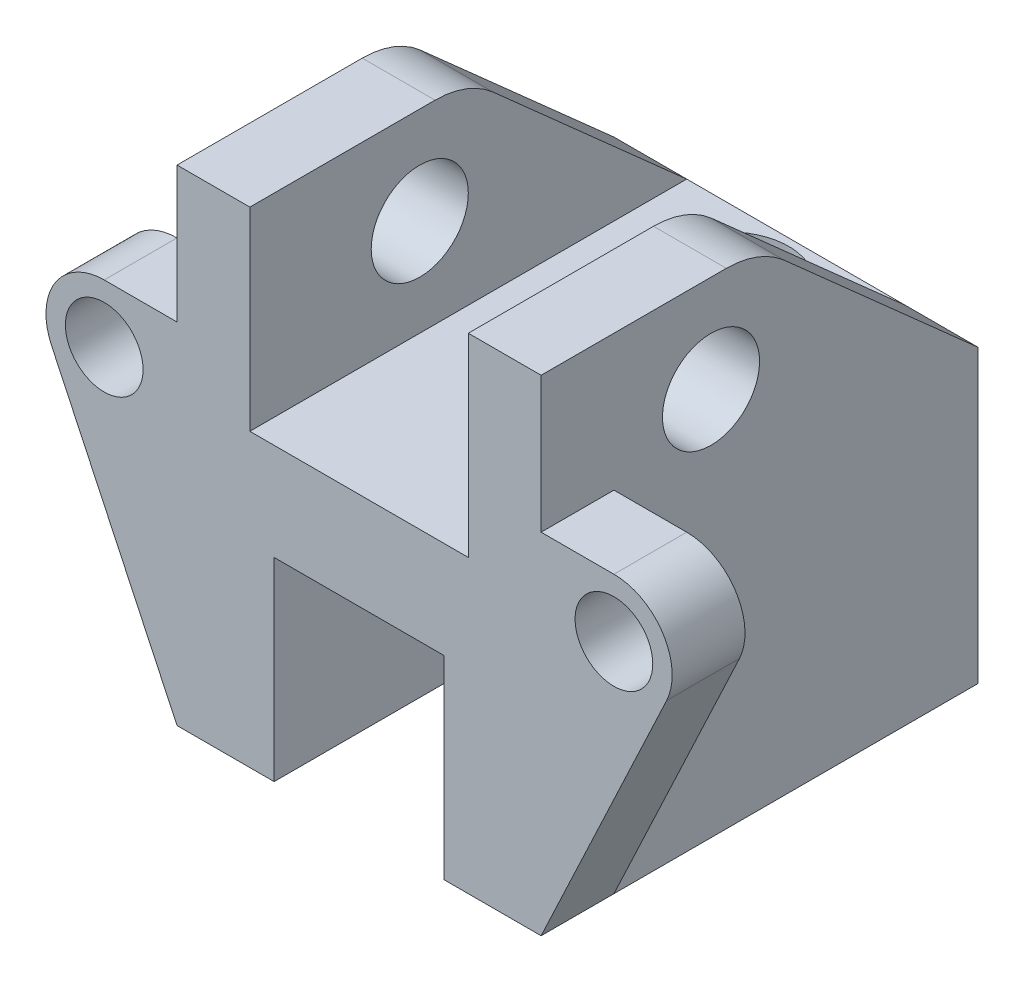
ISO-10303-21;
HEADER;
FILE_DESCRIPTION(('STEP AP214'),'2;1');
FILE_NAME('part.step','',(''),(''),'','','');
FILE_SCHEMA(('AUTOMOTIVE_DESIGN { 1 0 10303 214 1 1 1 1 }'));
ENDSEC;
DATA;
#1=APPLICATION_CONTEXT('core data for automotive mechanical design processes');
#2=APPLICATION_PROTOCOL_DEFINITION('international standard','automotive_design',2000,#1);
#3=PRODUCT_CONTEXT('',#1,'mechanical');
#4=PRODUCT('Part','Part','',(#3));
#5=PRODUCT_RELATED_PRODUCT_CATEGORY('part','',(#4));
#6=PRODUCT_DEFINITION_FORMATION('','',#4);
#7=PRODUCT_DEFINITION_CONTEXT('part definition',#1,'design');
#8=PRODUCT_DEFINITION('design','',#6,#7);
#9=PRODUCT_DEFINITION_SHAPE('','',#8);
#10=(LENGTH_UNIT() NAMED_UNIT(*) SI_UNIT(.MILLI.,.METRE.));
#11=(NAMED_UNIT(*) PLANE_ANGLE_UNIT() SI_UNIT($,.RADIAN.));
#12=(NAMED_UNIT(*) SI_UNIT($,.STERADIAN.) SOLID_ANGLE_UNIT());
#13=UNCERTAINTY_MEASURE_WITH_UNIT(LENGTH_MEASURE(1.E-05),#10,'distance_accuracy_value','');
#14=(GEOMETRIC_REPRESENTATION_CONTEXT(3) GLOBAL_UNCERTAINTY_ASSIGNED_CONTEXT((#13)) GLOBAL_UNIT_ASSIGNED_CONTEXT((#10,
#11,#12)) REPRESENTATION_CONTEXT('',''));
#15=CARTESIAN_POINT('',(0.,0.,0.));
#16=DIRECTION('',(0.,0.,1.));
#17=DIRECTION('',(1.,0.,0.));
#18=AXIS2_PLACEMENT_3D('',#15,#16,#17);
#19=CARTESIAN_POINT('',(-75.,0.,0.));
#20=DIRECTION('',(-1.,0.,0.));
#21=DIRECTION('',(0.,0.,1.));
#22=AXIS2_PLACEMENT_3D('',#19,#20,#21);
#23=PLANE('',#22);
#24=CARTESIAN_POINT('',(-75.,80.,-35.));
#25=DIRECTION('',(1.,0.,0.));
#26=DIRECTION('',(0.,0.,-1.));
#27=AXIS2_PLACEMENT_3D('',#24,#25,#26);
#28=CIRCLE('',#27,10.);
#29=CARTESIAN_POINT('',(-75.,80.,-45.));
#30=VERTEX_POINT('',#29);
#31=EDGE_CURVE('E275',#30,#30,#28,.T.);
#32=ORIENTED_EDGE('',*,*,#31,.T.);
#33=EDGE_LOOP('',(#32));
#34=FACE_BOUND('',#33,.T.);
#35=DIRECTION('',(0.,0.,-1.));
#36=VECTOR('',#35,1.);
#37=CARTESIAN_POINT('',(-75.,0.,0.));
#38=LINE('',#37,#36);
#39=CARTESIAN_POINT('',(-75.,0.,-15.));
#40=VERTEX_POINT('',#39);
#41=CARTESIAN_POINT('',(-75.,0.,-90.));
#42=VERTEX_POINT('',#41);
#43=EDGE_CURVE('E335',#40,#42,#38,.T.);
#44=ORIENTED_EDGE('',*,*,#43,.F.);
#45=DIRECTION('',(0.,1.,0.));
#46=VECTOR('',#45,1.);
#47=CARTESIAN_POINT('',(-75.,72.,-15.));
#48=LINE('',#47,#46);
#49=CARTESIAN_POINT('',(-75.,72.,-15.));
#50=VERTEX_POINT('',#49);
#51=EDGE_CURVE('E216',#40,#50,#48,.T.);
#52=ORIENTED_EDGE('',*,*,#51,.T.);
#53=DIRECTION('',(0.,0.,1.));
#54=VECTOR('',#53,1.);
#55=CARTESIAN_POINT('',(-75.,72.,-15.));
#56=LINE('',#55,#54);
#57=CARTESIAN_POINT('',(-75.,72.,0.));
#58=VERTEX_POINT('',#57);
#59=EDGE_CURVE('E206',#50,#58,#56,.T.);
#60=ORIENTED_EDGE('',*,*,#59,.T.);
#61=DIRECTION('',(0.,-1.,0.));
#62=VECTOR('',#61,1.);
#63=CARTESIAN_POINT('',(-75.,0.,0.));
#64=LINE('',#63,#62);
#65=CARTESIAN_POINT('',(-75.,100.,0.));
#66=VERTEX_POINT('',#65);
#67=EDGE_CURVE('E328',#66,#58,#64,.T.);
#68=ORIENTED_EDGE('',*,*,#67,.F.);
#69=DIRECTION('',(0.,0.,1.));
#70=VECTOR('',#69,1.);
#71=CARTESIAN_POINT('',(-75.,100.,0.));
#72=LINE('',#71,#70);
#73=CARTESIAN_POINT('',(-75.,100.,-38.1564121977173));
#74=VERTEX_POINT('',#73);
#75=EDGE_CURVE('E343',#74,#66,#72,.T.);
#76=ORIENTED_EDGE('',*,*,#75,.F.);
#77=CARTESIAN_POINT('',(-75.,82.,-38.1564121977173));
#78=DIRECTION('',(-1.,0.,0.));
#79=DIRECTION('',(0.,0.,1.));
#80=AXIS2_PLACEMENT_3D('',#77,#78,#79);
#81=CIRCLE('',#80,18.);
#82=CARTESIAN_POINT('',(-75.,95.4533677363059,-50.1149612966559));
#83=VERTEX_POINT('',#82);
#84=EDGE_CURVE('E11',#74,#83,#81,.T.);
#85=ORIENTED_EDGE('',*,*,#84,.T.);
#86=DIRECTION('',(0.,0.66436383882992,0.74740931868366));
#87=VECTOR('',#86,1.);
#88=CARTESIAN_POINT('',(-75.,100.,-45.));
#89=LINE('',#88,#87);
#90=CARTESIAN_POINT('',(-75.,60.,-90.));
#91=VERTEX_POINT('',#90);
#92=EDGE_CURVE('E338',#91,#83,#89,.T.);
#93=ORIENTED_EDGE('',*,*,#92,.F.);
#94=DIRECTION('',(0.,1.,0.));
#95=VECTOR('',#94,1.);
#96=CARTESIAN_POINT('',(-75.,0.,-90.));
#97=LINE('',#96,#95);
#98=EDGE_CURVE('E339',#42,#91,#97,.T.);
#99=ORIENTED_EDGE('',*,*,#98,.F.);
#100=EDGE_LOOP('',(#44,#52,#60,#68,#76,#85,#93,#99));
#101=FACE_BOUND('',#100,.T.);
#102=ADVANCED_FACE('F44',(#34,#101),#23,.T.);
#103=CARTESIAN_POINT('',(0.,0.,0.));
#104=DIRECTION('',(-1.,0.,0.));
#105=DIRECTION('',(0.,0.,1.));
#106=AXIS2_PLACEMENT_3D('',#103,#104,#105);
#107=PLANE('',#106);
#108=CARTESIAN_POINT('',(0.,80.,-35.));
#109=DIRECTION('',(1.,0.,0.));
#110=DIRECTION('',(0.,0.,-1.));
#111=AXIS2_PLACEMENT_3D('',#108,#109,#110);
#112=CIRCLE('',#111,10.);
#113=CARTESIAN_POINT('',(0.,80.,-45.));
#114=VERTEX_POINT('',#113);
#115=EDGE_CURVE('E271',#114,#114,#112,.T.);
#116=ORIENTED_EDGE('',*,*,#115,.F.);
#117=EDGE_LOOP('',(#116));
#118=FACE_BOUND('',#117,.T.);
#119=DIRECTION('',(0.,0.,1.));
#120=VECTOR('',#119,1.);
#121=CARTESIAN_POINT('',(0.,72.,-15.));
#122=LINE('',#121,#120);
#123=CARTESIAN_POINT('',(0.,72.,-15.));
#124=VERTEX_POINT('',#123);
#125=CARTESIAN_POINT('',(0.,72.,0.));
#126=VERTEX_POINT('',#125);
#127=EDGE_CURVE('E263',#124,#126,#122,.T.);
#128=ORIENTED_EDGE('',*,*,#127,.F.);
#129=DIRECTION('',(0.,-1.,0.));
#130=VECTOR('',#129,1.);
#131=CARTESIAN_POINT('',(0.,72.,-15.));
#132=LINE('',#131,#130);
#133=CARTESIAN_POINT('',(0.,0.,-15.));
#134=VERTEX_POINT('',#133);
#135=EDGE_CURVE('E248',#124,#134,#132,.T.);
#136=ORIENTED_EDGE('',*,*,#135,.T.);
#137=DIRECTION('',(0.,0.,-1.));
#138=VECTOR('',#137,1.);
#139=CARTESIAN_POINT('',(0.,0.,0.));
#140=LINE('',#139,#138);
#141=CARTESIAN_POINT('',(0.,0.,-90.));
#142=VERTEX_POINT('',#141);
#143=EDGE_CURVE('E346',#134,#142,#140,.T.);
#144=ORIENTED_EDGE('',*,*,#143,.T.);
#145=DIRECTION('',(0.,1.,0.));
#146=VECTOR('',#145,1.);
#147=CARTESIAN_POINT('',(0.,0.,-90.));
#148=LINE('',#147,#146);
#149=CARTESIAN_POINT('',(0.,60.,-90.));
#150=VERTEX_POINT('',#149);
#151=EDGE_CURVE('E352',#142,#150,#148,.T.);
#152=ORIENTED_EDGE('',*,*,#151,.T.);
#153=DIRECTION('',(0.,0.66436383882992,0.74740931868366));
#154=VECTOR('',#153,1.);
#155=CARTESIAN_POINT('',(0.,100.,-45.));
#156=LINE('',#155,#154);
#157=CARTESIAN_POINT('',(0.,95.4533677363059,-50.1149612966559));
#158=VERTEX_POINT('',#157);
#159=EDGE_CURVE('E351',#150,#158,#156,.T.);
#160=ORIENTED_EDGE('',*,*,#159,.T.);
#161=CARTESIAN_POINT('',(0.,82.,-38.1564121977173));
#162=DIRECTION('',(-1.,0.,0.));
#163=DIRECTION('',(0.,0.,1.));
#164=AXIS2_PLACEMENT_3D('',#161,#162,#163);
#165=CIRCLE('',#164,18.);
#166=CARTESIAN_POINT('',(0.,100.,-38.1564121977173));
#167=VERTEX_POINT('',#166);
#168=EDGE_CURVE('E381',#158,#167,#165,.F.);
#169=ORIENTED_EDGE('',*,*,#168,.T.);
#170=DIRECTION('',(0.,0.,1.));
#171=VECTOR('',#170,1.);
#172=CARTESIAN_POINT('',(0.,100.,0.));
#173=LINE('',#172,#171);
#174=CARTESIAN_POINT('',(0.,100.,0.));
#175=VERTEX_POINT('',#174);
#176=EDGE_CURVE('E334',#167,#175,#173,.T.);
#177=ORIENTED_EDGE('',*,*,#176,.T.);
#178=DIRECTION('',(0.,-1.,0.));
#179=VECTOR('',#178,1.);
#180=CARTESIAN_POINT('',(0.,0.,0.));
#181=LINE('',#180,#179);
#182=EDGE_CURVE('E325',#175,#126,#181,.T.);
#183=ORIENTED_EDGE('',*,*,#182,.T.);
#184=EDGE_LOOP('',(#128,#136,#144,#152,#160,#169,#177,#183));
#185=FACE_BOUND('',#184,.T.);
#186=ADVANCED_FACE('F450',(#118,#185),#107,.F.);
#187=CARTESIAN_POINT('',(-75.,100.,0.));
#188=DIRECTION('',(0.,1.,0.));
#189=DIRECTION('',(0.,0.,1.));
#190=AXIS2_PLACEMENT_3D('',#187,#188,#189);
#191=PLANE('',#190);
#192=DIRECTION('',(0.,0.,1.));
#193=VECTOR('',#192,1.);
#194=CARTESIAN_POINT('',(-60.,100.,0.));
#195=LINE('',#194,#193);
#196=CARTESIAN_POINT('',(-60.,100.,-38.1564121977173));
#197=VERTEX_POINT('',#196);
#198=CARTESIAN_POINT('',(-60.,100.,0.));
#199=VERTEX_POINT('',#198);
#200=EDGE_CURVE('E278',#197,#199,#195,.T.);
#201=ORIENTED_EDGE('',*,*,#200,.F.);
#202=DIRECTION('',(1.,0.,0.));
#203=VECTOR('',#202,1.);
#204=CARTESIAN_POINT('',(-75.,100.,-38.1564121977173));
#205=LINE('',#204,#203);
#206=EDGE_CURVE('E53',#197,#74,#205,.F.);
#207=ORIENTED_EDGE('',*,*,#206,.T.);
#208=ORIENTED_EDGE('',*,*,#75,.T.);
#209=DIRECTION('',(1.,0.,0.));
#210=VECTOR('',#209,1.);
#211=CARTESIAN_POINT('',(-75.,100.,0.));
#212=LINE('',#211,#210);
#213=EDGE_CURVE('E358',#66,#199,#212,.T.);
#214=ORIENTED_EDGE('',*,*,#213,.T.);
#215=EDGE_LOOP('',(#201,#207,#208,#214));
#216=FACE_BOUND('',#215,.T.);
#217=ADVANCED_FACE('F396',(#216),#191,.T.);
#218=CARTESIAN_POINT('',(-75.,100.,-45.));
#219=DIRECTION('',(0.,0.74740931868366,-0.66436383882992));
#220=DIRECTION('',(0.,0.66436383882992,0.74740931868366));
#221=AXIS2_PLACEMENT_3D('',#218,#219,#220);
#222=PLANE('',#221);
#223=ORIENTED_EDGE('',*,*,#92,.T.);
#224=DIRECTION('',(1.,0.,0.));
#225=VECTOR('',#224,1.);
#226=CARTESIAN_POINT('',(-75.,95.4533677363059,-50.1149612966559));
#227=LINE('',#226,#225);
#228=CARTESIAN_POINT('',(-60.,95.4533677363059,-50.1149612966559));
#229=VERTEX_POINT('',#228);
#230=EDGE_CURVE('E390',#83,#229,#227,.T.);
#231=ORIENTED_EDGE('',*,*,#230,.T.);
#232=DIRECTION('',(0.,0.66436383882992,0.74740931868366));
#233=VECTOR('',#232,1.);
#234=CARTESIAN_POINT('',(-60.,100.,-45.));
#235=LINE('',#234,#233);
#236=CARTESIAN_POINT('',(-60.,60.,-90.));
#237=VERTEX_POINT('',#236);
#238=EDGE_CURVE('E374',#237,#229,#235,.T.);
#239=ORIENTED_EDGE('',*,*,#238,.F.);
#240=DIRECTION('',(1.,0.,0.));
#241=VECTOR('',#240,1.);
#242=CARTESIAN_POINT('',(-75.,60.,-90.));
#243=LINE('',#242,#241);
#244=EDGE_CURVE('E361',#91,#237,#243,.T.);
#245=ORIENTED_EDGE('',*,*,#244,.F.);
#246=EDGE_LOOP('',(#223,#231,#239,#245));
#247=FACE_BOUND('',#246,.T.);
#248=ADVANCED_FACE('F407',(#247),#222,.T.);
#249=CARTESIAN_POINT('',(-75.,0.,0.));
#250=DIRECTION('',(0.,-1.,0.));
#251=DIRECTION('',(0.,0.,-1.));
#252=AXIS2_PLACEMENT_3D('',#249,#250,#251);
#253=PLANE('',#252);
#254=DIRECTION('',(0.,0.,-1.));
#255=VECTOR('',#254,1.);
#256=CARTESIAN_POINT('',(-20.,0.,0.));
#257=LINE('',#256,#255);
#258=CARTESIAN_POINT('',(-20.,0.,0.));
#259=VERTEX_POINT('',#258);
#260=CARTESIAN_POINT('',(-20.,0.,-90.));
#261=VERTEX_POINT('',#260);
#262=EDGE_CURVE('E311',#259,#261,#257,.T.);
#263=ORIENTED_EDGE('',*,*,#262,.T.);
#264=DIRECTION('',(1.,0.,0.));
#265=VECTOR('',#264,1.);
#266=CARTESIAN_POINT('',(-75.,0.,-90.));
#267=LINE('',#266,#265);
#268=EDGE_CURVE('E367',#261,#142,#267,.T.);
#269=ORIENTED_EDGE('',*,*,#268,.T.);
#270=ORIENTED_EDGE('',*,*,#143,.F.);
#271=CARTESIAN_POINT('',(0.,0.,0.));
#272=VERTEX_POINT('',#271);
#273=EDGE_CURVE('E349',#272,#134,#140,.T.);
#274=ORIENTED_EDGE('',*,*,#273,.F.);
#275=DIRECTION('',(1.,0.,0.));
#276=VECTOR('',#275,1.);
#277=CARTESIAN_POINT('',(-75.,0.,0.));
#278=LINE('',#277,#276);
#279=EDGE_CURVE('E344',#259,#272,#278,.T.);
#280=ORIENTED_EDGE('',*,*,#279,.F.);
#281=EDGE_LOOP('',(#263,#269,#270,#274,#280));
#282=FACE_BOUND('',#281,.T.);
#283=ADVANCED_FACE('F452',(#282),#253,.T.);
#284=CARTESIAN_POINT('',(-75.,0.,0.));
#285=DIRECTION('',(0.,0.,1.));
#286=DIRECTION('',(1.,0.,0.));
#287=AXIS2_PLACEMENT_3D('',#284,#285,#286);
#288=PLANE('',#287);
#289=DIRECTION('',(0.,1.,0.));
#290=VECTOR('',#289,1.);
#291=CARTESIAN_POINT('',(-60.,60.,0.));
#292=LINE('',#291,#290);
#293=CARTESIAN_POINT('',(-60.,60.,0.));
#294=VERTEX_POINT('',#293);
#295=EDGE_CURVE('E294',#294,#199,#292,.T.);
#296=ORIENTED_EDGE('',*,*,#295,.T.);
#297=ORIENTED_EDGE('',*,*,#213,.F.);
#298=ORIENTED_EDGE('',*,*,#67,.T.);
#299=DIRECTION('',(-1.,0.,0.));
#300=VECTOR('',#299,1.);
#301=CARTESIAN_POINT('',(-90.,72.,0.));
#302=LINE('',#301,#300);
#303=CARTESIAN_POINT('',(-90.,72.,0.));
#304=VERTEX_POINT('',#303);
#305=EDGE_CURVE('E62',#58,#304,#302,.T.);
#306=ORIENTED_EDGE('',*,*,#305,.T.);
#307=CARTESIAN_POINT('',(-90.,60.,0.));
#308=DIRECTION('',(0.,0.,1.));
#309=DIRECTION('',(1.,0.,0.));
#310=AXIS2_PLACEMENT_3D('',#307,#308,#309);
#311=CIRCLE('',#310,12.);
#312=CARTESIAN_POINT('',(-100.855763811477,54.8860590471308,0.));
#313=VERTEX_POINT('',#312);
#314=EDGE_CURVE('E230',#304,#313,#311,.T.);
#315=ORIENTED_EDGE('',*,*,#314,.T.);
#316=DIRECTION('',(0.426161746072432,-0.904646984289726,0.));
#317=VECTOR('',#316,1.);
#318=CARTESIAN_POINT('',(-75.,0.,0.));
#319=LINE('',#318,#317);
#320=CARTESIAN_POINT('',(-75.,0.,0.));
#321=VERTEX_POINT('',#320);
#322=EDGE_CURVE('E203',#313,#321,#319,.T.);
#323=ORIENTED_EDGE('',*,*,#322,.T.);
#324=CARTESIAN_POINT('',(-55.,0.,0.));
#325=VERTEX_POINT('',#324);
#326=EDGE_CURVE('E371',#321,#325,#278,.T.);
#327=ORIENTED_EDGE('',*,*,#326,.T.);
#328=DIRECTION('',(0.,1.,0.));
#329=VECTOR('',#328,1.);
#330=CARTESIAN_POINT('',(-55.,0.,0.));
#331=LINE('',#330,#329);
#332=CARTESIAN_POINT('',(-55.,40.,0.));
#333=VERTEX_POINT('',#332);
#334=EDGE_CURVE('E308',#325,#333,#331,.T.);
#335=ORIENTED_EDGE('',*,*,#334,.T.);
#336=DIRECTION('',(1.,0.,0.));
#337=VECTOR('',#336,1.);
#338=CARTESIAN_POINT('',(-20.,40.,0.));
#339=LINE('',#338,#337);
#340=CARTESIAN_POINT('',(-20.,40.,0.));
#341=VERTEX_POINT('',#340);
#342=EDGE_CURVE('E309',#333,#341,#339,.T.);
#343=ORIENTED_EDGE('',*,*,#342,.T.);
#344=DIRECTION('',(0.,-1.,0.));
#345=VECTOR('',#344,1.);
#346=CARTESIAN_POINT('',(-20.,0.,0.));
#347=LINE('',#346,#345);
#348=EDGE_CURVE('E303',#341,#259,#347,.T.);
#349=ORIENTED_EDGE('',*,*,#348,.T.);
#350=ORIENTED_EDGE('',*,*,#279,.T.);
#351=DIRECTION('',(0.426161746072432,0.904646984289726,0.));
#352=VECTOR('',#351,1.);
#353=CARTESIAN_POINT('',(0.,0.,0.));
#354=LINE('',#353,#352);
#355=CARTESIAN_POINT('',(25.8557638114767,54.8860590471308,0.));
#356=VERTEX_POINT('',#355);
#357=EDGE_CURVE('E243',#272,#356,#354,.T.);
#358=ORIENTED_EDGE('',*,*,#357,.T.);
#359=CARTESIAN_POINT('',(15.,60.,0.));
#360=DIRECTION('',(0.,0.,1.));
#361=DIRECTION('',(1.,0.,0.));
#362=AXIS2_PLACEMENT_3D('',#359,#360,#361);
#363=CIRCLE('',#362,12.);
#364=CARTESIAN_POINT('',(15.,72.,0.));
#365=VERTEX_POINT('',#364);
#366=EDGE_CURVE('E236',#356,#365,#363,.T.);
#367=ORIENTED_EDGE('',*,*,#366,.T.);
#368=DIRECTION('',(-1.,0.,0.));
#369=VECTOR('',#368,1.);
#370=CARTESIAN_POINT('',(15.,72.,0.));
#371=LINE('',#370,#369);
#372=EDGE_CURVE('E254',#365,#126,#371,.T.);
#373=ORIENTED_EDGE('',*,*,#372,.T.);
#374=ORIENTED_EDGE('',*,*,#182,.F.);
#375=CARTESIAN_POINT('',(-15.,100.,0.));
#376=VERTEX_POINT('',#375);
#377=EDGE_CURVE('E362',#376,#175,#212,.T.);
#378=ORIENTED_EDGE('',*,*,#377,.F.);
#379=DIRECTION('',(0.,1.,0.));
#380=VECTOR('',#379,1.);
#381=CARTESIAN_POINT('',(-15.,60.,0.));
#382=LINE('',#381,#380);
#383=CARTESIAN_POINT('',(-15.,60.,0.));
#384=VERTEX_POINT('',#383);
#385=EDGE_CURVE('E300',#384,#376,#382,.T.);
#386=ORIENTED_EDGE('',*,*,#385,.F.);
#387=DIRECTION('',(1.,0.,0.));
#388=VECTOR('',#387,1.);
#389=CARTESIAN_POINT('',(-60.,60.,0.));
#390=LINE('',#389,#388);
#391=EDGE_CURVE('E281',#294,#384,#390,.T.);
#392=ORIENTED_EDGE('',*,*,#391,.F.);
#393=EDGE_LOOP('',(#296,#297,#298,#306,#315,#323,#327,#335,#343,#349,#350,#358,#367,#373,#374,
#378,#386,#392));
#394=FACE_BOUND('',#393,.T.);
#395=CARTESIAN_POINT('',(15.,60.,0.));
#396=DIRECTION('',(0.,0.,1.));
#397=DIRECTION('',(1.,0.,0.));
#398=AXIS2_PLACEMENT_3D('',#395,#396,#397);
#399=CIRCLE('',#398,8.);
#400=CARTESIAN_POINT('',(23.,60.,0.));
#401=VERTEX_POINT('',#400);
#402=EDGE_CURVE('E233',#401,#401,#399,.T.);
#403=ORIENTED_EDGE('',*,*,#402,.F.);
#404=EDGE_LOOP('',(#403));
#405=FACE_BOUND('',#404,.T.);
#406=CARTESIAN_POINT('',(-90.,60.,0.));
#407=DIRECTION('',(0.,0.,1.));
#408=DIRECTION('',(1.,0.,0.));
#409=AXIS2_PLACEMENT_3D('',#406,#407,#408);
#410=CIRCLE('',#409,8.00000000000001);
#411=CARTESIAN_POINT('',(-82.,60.,0.));
#412=VERTEX_POINT('',#411);
#413=EDGE_CURVE('E224',#412,#412,#410,.T.);
#414=ORIENTED_EDGE('',*,*,#413,.F.);
#415=EDGE_LOOP('',(#414));
#416=FACE_BOUND('',#415,.T.);
#417=ADVANCED_FACE('F426',(#394,#405,#416),#288,.T.);
#418=ORIENTED_EDGE('',*,*,#176,.F.);
#419=DIRECTION('',(1.,0.,0.));
#420=VECTOR('',#419,1.);
#421=CARTESIAN_POINT('',(-75.,100.,-38.1564121977173));
#422=LINE('',#421,#420);
#423=CARTESIAN_POINT('',(-15.,100.,-38.1564121977173));
#424=VERTEX_POINT('',#423);
#425=EDGE_CURVE('E382',#167,#424,#422,.F.);
#426=ORIENTED_EDGE('',*,*,#425,.T.);
#427=DIRECTION('',(0.,0.,-1.));
#428=VECTOR('',#427,1.);
#429=CARTESIAN_POINT('',(-15.,100.,0.));
#430=LINE('',#429,#428);
#431=EDGE_CURVE('E283',#376,#424,#430,.T.);
#432=ORIENTED_EDGE('',*,*,#431,.F.);
#433=ORIENTED_EDGE('',*,*,#377,.T.);
#434=EDGE_LOOP('',(#418,#426,#432,#433));
#435=FACE_BOUND('',#434,.T.);
#436=ADVANCED_FACE('F437',(#435),#191,.T.);
#437=DIRECTION('',(0.,-0.66436383882992,-0.74740931868366));
#438=VECTOR('',#437,1.);
#439=CARTESIAN_POINT('',(-15.,100.,-45.));
#440=LINE('',#439,#438);
#441=CARTESIAN_POINT('',(-15.,95.4533677363059,-50.1149612966559));
#442=VERTEX_POINT('',#441);
#443=CARTESIAN_POINT('',(-15.,60.,-90.));
#444=VERTEX_POINT('',#443);
#445=EDGE_CURVE('E363',#442,#444,#440,.T.);
#446=ORIENTED_EDGE('',*,*,#445,.F.);
#447=DIRECTION('',(1.,0.,0.));
#448=VECTOR('',#447,1.);
#449=CARTESIAN_POINT('',(-75.,95.4533677363059,-50.1149612966559));
#450=LINE('',#449,#448);
#451=EDGE_CURVE('E378',#442,#158,#450,.T.);
#452=ORIENTED_EDGE('',*,*,#451,.T.);
#453=ORIENTED_EDGE('',*,*,#159,.F.);
#454=EDGE_CURVE('E368',#444,#150,#243,.T.);
#455=ORIENTED_EDGE('',*,*,#454,.F.);
#456=EDGE_LOOP('',(#446,#452,#453,#455));
#457=FACE_BOUND('',#456,.T.);
#458=ADVANCED_FACE('F443',(#457),#222,.T.);
#459=CARTESIAN_POINT('',(-75.,0.,-90.));
#460=DIRECTION('',(0.,0.,-1.));
#461=DIRECTION('',(-1.,0.,0.));
#462=AXIS2_PLACEMENT_3D('',#459,#460,#461);
#463=PLANE('',#462);
#464=DIRECTION('',(0.,-1.,0.));
#465=VECTOR('',#464,1.);
#466=CARTESIAN_POINT('',(-20.,0.,-90.));
#467=LINE('',#466,#465);
#468=CARTESIAN_POINT('',(-20.,40.,-90.));
#469=VERTEX_POINT('',#468);
#470=EDGE_CURVE('E298',#469,#261,#467,.T.);
#471=ORIENTED_EDGE('',*,*,#470,.F.);
#472=DIRECTION('',(1.,0.,0.));
#473=VECTOR('',#472,1.);
#474=CARTESIAN_POINT('',(-20.,40.,-90.));
#475=LINE('',#474,#473);
#476=CARTESIAN_POINT('',(-55.,40.,-90.));
#477=VERTEX_POINT('',#476);
#478=EDGE_CURVE('E307',#477,#469,#475,.T.);
#479=ORIENTED_EDGE('',*,*,#478,.F.);
#480=DIRECTION('',(0.,1.,0.));
#481=VECTOR('',#480,1.);
#482=CARTESIAN_POINT('',(-55.,0.,-90.));
#483=LINE('',#482,#481);
#484=CARTESIAN_POINT('',(-55.,0.,-90.));
#485=VERTEX_POINT('',#484);
#486=EDGE_CURVE('E312',#485,#477,#483,.T.);
#487=ORIENTED_EDGE('',*,*,#486,.F.);
#488=EDGE_CURVE('E370',#42,#485,#267,.T.);
#489=ORIENTED_EDGE('',*,*,#488,.F.);
#490=ORIENTED_EDGE('',*,*,#98,.T.);
#491=ORIENTED_EDGE('',*,*,#244,.T.);
#492=DIRECTION('',(-1.,0.,0.));
#493=VECTOR('',#492,1.);
#494=CARTESIAN_POINT('',(-60.,60.,-90.));
#495=LINE('',#494,#493);
#496=EDGE_CURVE('E292',#444,#237,#495,.T.);
#497=ORIENTED_EDGE('',*,*,#496,.F.);
#498=ORIENTED_EDGE('',*,*,#454,.T.);
#499=ORIENTED_EDGE('',*,*,#151,.F.);
#500=ORIENTED_EDGE('',*,*,#268,.F.);
#501=EDGE_LOOP('',(#471,#479,#487,#489,#490,#491,#497,#498,#499,#500));
#502=FACE_BOUND('',#501,.T.);
#503=ADVANCED_FACE('F418',(#502),#463,.T.);
#504=DIRECTION('',(0.,0.,-1.));
#505=VECTOR('',#504,1.);
#506=CARTESIAN_POINT('',(-55.,0.,0.));
#507=LINE('',#506,#505);
#508=EDGE_CURVE('E324',#325,#485,#507,.T.);
#509=ORIENTED_EDGE('',*,*,#508,.F.);
#510=ORIENTED_EDGE('',*,*,#326,.F.);
#511=EDGE_CURVE('E331',#321,#40,#38,.T.);
#512=ORIENTED_EDGE('',*,*,#511,.T.);
#513=ORIENTED_EDGE('',*,*,#43,.T.);
#514=ORIENTED_EDGE('',*,*,#488,.T.);
#515=EDGE_LOOP('',(#509,#510,#512,#513,#514));
#516=FACE_BOUND('',#515,.T.);
#517=ADVANCED_FACE('F424',(#516),#253,.T.);
#518=CARTESIAN_POINT('',(-20.,0.,0.));
#519=DIRECTION('',(1.,0.,0.));
#520=DIRECTION('',(0.,0.,-1.));
#521=AXIS2_PLACEMENT_3D('',#518,#519,#520);
#522=PLANE('',#521);
#523=ORIENTED_EDGE('',*,*,#470,.T.);
#524=ORIENTED_EDGE('',*,*,#262,.F.);
#525=ORIENTED_EDGE('',*,*,#348,.F.);
#526=DIRECTION('',(0.,0.,-1.));
#527=VECTOR('',#526,1.);
#528=CARTESIAN_POINT('',(-20.,40.,0.));
#529=LINE('',#528,#527);
#530=EDGE_CURVE('E319',#341,#469,#529,.T.);
#531=ORIENTED_EDGE('',*,*,#530,.T.);
#532=EDGE_LOOP('',(#523,#524,#525,#531));
#533=FACE_BOUND('',#532,.T.);
#534=ADVANCED_FACE('F458',(#533),#522,.F.);
#535=CARTESIAN_POINT('',(-20.,40.,0.));
#536=DIRECTION('',(0.,1.,0.));
#537=DIRECTION('',(0.,0.,1.));
#538=AXIS2_PLACEMENT_3D('',#535,#536,#537);
#539=PLANE('',#538);
#540=CARTESIAN_POINT('',(-37.5,40.,-76.));
#541=DIRECTION('',(0.,1.,0.));
#542=DIRECTION('',(0.,0.,1.));
#543=AXIS2_PLACEMENT_3D('',#540,#541,#542);
#544=CIRCLE('',#543,12.5);
#545=CARTESIAN_POINT('',(-37.5,40.,-63.5));
#546=VERTEX_POINT('',#545);
#547=EDGE_CURVE('E268',#546,#546,#544,.T.);
#548=ORIENTED_EDGE('',*,*,#547,.T.);
#549=EDGE_LOOP('',(#548));
#550=FACE_BOUND('',#549,.T.);
#551=ORIENTED_EDGE('',*,*,#478,.T.);
#552=ORIENTED_EDGE('',*,*,#530,.F.);
#553=ORIENTED_EDGE('',*,*,#342,.F.);
#554=DIRECTION('',(0.,0.,-1.));
#555=VECTOR('',#554,1.);
#556=CARTESIAN_POINT('',(-55.,40.,0.));
#557=LINE('',#556,#555);
#558=EDGE_CURVE('E323',#333,#477,#557,.T.);
#559=ORIENTED_EDGE('',*,*,#558,.T.);
#560=EDGE_LOOP('',(#551,#552,#553,#559));
#561=FACE_BOUND('',#560,.T.);
#562=ADVANCED_FACE('F465',(#550,#561),#539,.F.);
#563=CARTESIAN_POINT('',(-55.,0.,0.));
#564=DIRECTION('',(-1.,0.,0.));
#565=DIRECTION('',(0.,0.,1.));
#566=AXIS2_PLACEMENT_3D('',#563,#564,#565);
#567=PLANE('',#566);
#568=ORIENTED_EDGE('',*,*,#486,.T.);
#569=ORIENTED_EDGE('',*,*,#558,.F.);
#570=ORIENTED_EDGE('',*,*,#334,.F.);
#571=ORIENTED_EDGE('',*,*,#508,.T.);
#572=EDGE_LOOP('',(#568,#569,#570,#571));
#573=FACE_BOUND('',#572,.T.);
#574=ADVANCED_FACE('F466',(#573),#567,.F.);
#575=CARTESIAN_POINT('',(-60.,60.,0.));
#576=DIRECTION('',(-1.,0.,0.));
#577=DIRECTION('',(0.,0.,1.));
#578=AXIS2_PLACEMENT_3D('',#575,#576,#577);
#579=PLANE('',#578);
#580=CARTESIAN_POINT('',(-60.,80.,-35.));
#581=DIRECTION('',(-1.,0.,0.));
#582=DIRECTION('',(0.,0.,1.));
#583=AXIS2_PLACEMENT_3D('',#580,#581,#582);
#584=CIRCLE('',#583,10.);
#585=CARTESIAN_POINT('',(-60.,80.,-25.));
#586=VERTEX_POINT('',#585);
#587=EDGE_CURVE('E280',#586,#586,#584,.T.);
#588=ORIENTED_EDGE('',*,*,#587,.T.);
#589=EDGE_LOOP('',(#588));
#590=FACE_BOUND('',#589,.T.);
#591=ORIENTED_EDGE('',*,*,#238,.T.);
#592=CARTESIAN_POINT('',(-60.,82.,-38.1564121977173));
#593=DIRECTION('',(-1.,0.,0.));
#594=DIRECTION('',(0.,0.,1.));
#595=AXIS2_PLACEMENT_3D('',#592,#593,#594);
#596=CIRCLE('',#595,18.);
#597=EDGE_CURVE('E388',#229,#197,#596,.F.);
#598=ORIENTED_EDGE('',*,*,#597,.T.);
#599=ORIENTED_EDGE('',*,*,#200,.T.);
#600=ORIENTED_EDGE('',*,*,#295,.F.);
#601=DIRECTION('',(0.,0.,1.));
#602=VECTOR('',#601,1.);
#603=CARTESIAN_POINT('',(-60.,60.,0.));
#604=LINE('',#603,#602);
#605=EDGE_CURVE('E282',#237,#294,#604,.T.);
#606=ORIENTED_EDGE('',*,*,#605,.F.);
#607=EDGE_LOOP('',(#591,#598,#599,#600,#606));
#608=FACE_BOUND('',#607,.T.);
#609=ADVANCED_FACE('F410',(#590,#608),#579,.F.);
#610=CARTESIAN_POINT('',(-15.,60.,0.));
#611=DIRECTION('',(1.,0.,0.));
#612=DIRECTION('',(0.,0.,-1.));
#613=AXIS2_PLACEMENT_3D('',#610,#611,#612);
#614=PLANE('',#613);
#615=CARTESIAN_POINT('',(-15.,80.,-35.));
#616=DIRECTION('',(1.,0.,0.));
#617=DIRECTION('',(0.,0.,-1.));
#618=AXIS2_PLACEMENT_3D('',#615,#616,#617);
#619=CIRCLE('',#618,10.);
#620=CARTESIAN_POINT('',(-15.,80.,-45.));
#621=VERTEX_POINT('',#620);
#622=EDGE_CURVE('E47',#621,#621,#619,.T.);
#623=ORIENTED_EDGE('',*,*,#622,.T.);
#624=EDGE_LOOP('',(#623));
#625=FACE_BOUND('',#624,.T.);
#626=ORIENTED_EDGE('',*,*,#431,.T.);
#627=CARTESIAN_POINT('',(-15.,82.,-38.1564121977173));
#628=DIRECTION('',(1.,0.,0.));
#629=DIRECTION('',(0.,0.,-1.));
#630=AXIS2_PLACEMENT_3D('',#627,#628,#629);
#631=CIRCLE('',#630,18.);
#632=EDGE_CURVE('E384',#424,#442,#631,.F.);
#633=ORIENTED_EDGE('',*,*,#632,.T.);
#634=ORIENTED_EDGE('',*,*,#445,.T.);
#635=DIRECTION('',(0.,0.,-1.));
#636=VECTOR('',#635,1.);
#637=CARTESIAN_POINT('',(-15.,60.,0.));
#638=LINE('',#637,#636);
#639=EDGE_CURVE('E288',#384,#444,#638,.T.);
#640=ORIENTED_EDGE('',*,*,#639,.F.);
#641=ORIENTED_EDGE('',*,*,#385,.T.);
#642=EDGE_LOOP('',(#626,#633,#634,#640,#641));
#643=FACE_BOUND('',#642,.T.);
#644=ADVANCED_FACE('F432',(#625,#643),#614,.F.);
#645=CARTESIAN_POINT('',(0.,60.,0.));
#646=DIRECTION('',(0.,-1.,0.));
#647=DIRECTION('',(0.,0.,-1.));
#648=AXIS2_PLACEMENT_3D('',#645,#646,#647);
#649=PLANE('',#648);
#650=CARTESIAN_POINT('',(-37.5,60.,-76.));
#651=DIRECTION('',(0.,1.,0.));
#652=DIRECTION('',(0.,0.,1.));
#653=AXIS2_PLACEMENT_3D('',#650,#651,#652);
#654=CIRCLE('',#653,12.5);
#655=CARTESIAN_POINT('',(-37.5,60.,-63.5));
#656=VERTEX_POINT('',#655);
#657=EDGE_CURVE('E265',#656,#656,#654,.T.);
#658=ORIENTED_EDGE('',*,*,#657,.F.);
#659=EDGE_LOOP('',(#658));
#660=FACE_BOUND('',#659,.T.);
#661=ORIENTED_EDGE('',*,*,#605,.T.);
#662=ORIENTED_EDGE('',*,*,#391,.T.);
#663=ORIENTED_EDGE('',*,*,#639,.T.);
#664=ORIENTED_EDGE('',*,*,#496,.T.);
#665=EDGE_LOOP('',(#661,#662,#663,#664));
#666=FACE_BOUND('',#665,.T.);
#667=ADVANCED_FACE('F415',(#660,#666),#649,.F.);
#668=CARTESIAN_POINT('',(-75.,82.,-38.1564121977173));
#669=DIRECTION('',(1.,0.,0.));
#670=DIRECTION('',(0.,0.,-1.));
#671=AXIS2_PLACEMENT_3D('',#668,#669,#670);
#672=CYLINDRICAL_SURFACE('',#671,18.);
#673=ORIENTED_EDGE('',*,*,#632,.F.);
#674=ORIENTED_EDGE('',*,*,#425,.F.);
#675=ORIENTED_EDGE('',*,*,#168,.F.);
#676=ORIENTED_EDGE('',*,*,#451,.F.);
#677=EDGE_LOOP('',(#673,#674,#675,#676));
#678=FACE_BOUND('',#677,.T.);
#679=ADVANCED_FACE('F442',(#678),#672,.T.);
#680=CARTESIAN_POINT('',(-75.,82.,-38.1564121977173));
#681=DIRECTION('',(1.,0.,0.));
#682=DIRECTION('',(0.,0.,-1.));
#683=AXIS2_PLACEMENT_3D('',#680,#681,#682);
#684=CYLINDRICAL_SURFACE('',#683,18.);
#685=ORIENTED_EDGE('',*,*,#84,.F.);
#686=ORIENTED_EDGE('',*,*,#206,.F.);
#687=ORIENTED_EDGE('',*,*,#597,.F.);
#688=ORIENTED_EDGE('',*,*,#230,.F.);
#689=EDGE_LOOP('',(#685,#686,#687,#688));
#690=FACE_BOUND('',#689,.T.);
#691=ADVANCED_FACE('F50',(#690),#684,.T.);
#692=CARTESIAN_POINT('',(-75.,80.,-35.));
#693=DIRECTION('',(1.,0.,0.));
#694=DIRECTION('',(0.,0.,-1.));
#695=AXIS2_PLACEMENT_3D('',#692,#693,#694);
#696=CYLINDRICAL_SURFACE('',#695,10.);
#697=ORIENTED_EDGE('',*,*,#115,.T.);
#698=EDGE_LOOP('',(#697));
#699=FACE_BOUND('',#698,.T.);
#700=ORIENTED_EDGE('',*,*,#622,.F.);
#701=EDGE_LOOP('',(#700));
#702=FACE_BOUND('',#701,.T.);
#703=ADVANCED_FACE('F505',(#699,#702),#696,.F.);
#704=ORIENTED_EDGE('',*,*,#31,.F.);
#705=EDGE_LOOP('',(#704));
#706=FACE_BOUND('',#705,.T.);
#707=ORIENTED_EDGE('',*,*,#587,.F.);
#708=EDGE_LOOP('',(#707));
#709=FACE_BOUND('',#708,.T.);
#710=ADVANCED_FACE('F514',(#706,#709),#696,.F.);
#711=CARTESIAN_POINT('',(-37.5,20.,-76.));
#712=DIRECTION('',(0.,1.,0.));
#713=DIRECTION('',(0.,0.,1.));
#714=AXIS2_PLACEMENT_3D('',#711,#712,#713);
#715=CYLINDRICAL_SURFACE('',#714,12.5);
#716=ORIENTED_EDGE('',*,*,#657,.T.);
#717=EDGE_LOOP('',(#716));
#718=FACE_BOUND('',#717,.T.);
#719=ORIENTED_EDGE('',*,*,#547,.F.);
#720=EDGE_LOOP('',(#719));
#721=FACE_BOUND('',#720,.T.);
#722=ADVANCED_FACE('F519',(#718,#721),#715,.F.);
#723=CARTESIAN_POINT('',(15.,60.,-15.));
#724=DIRECTION('',(0.,0.,1.));
#725=DIRECTION('',(1.,0.,0.));
#726=AXIS2_PLACEMENT_3D('',#723,#724,#725);
#727=CYLINDRICAL_SURFACE('',#726,12.);
#728=ORIENTED_EDGE('',*,*,#366,.F.);
#729=DIRECTION('',(0.,0.,1.));
#730=VECTOR('',#729,1.);
#731=CARTESIAN_POINT('',(25.8557638114767,54.8860590471308,-15.));
#732=LINE('',#731,#730);
#733=CARTESIAN_POINT('',(25.8557638114767,54.8860590471308,-15.));
#734=VERTEX_POINT('',#733);
#735=EDGE_CURVE('E257',#734,#356,#732,.T.);
#736=ORIENTED_EDGE('',*,*,#735,.F.);
#737=CARTESIAN_POINT('',(15.,60.,-15.));
#738=DIRECTION('',(0.,0.,1.));
#739=DIRECTION('',(1.,0.,0.));
#740=AXIS2_PLACEMENT_3D('',#737,#738,#739);
#741=CIRCLE('',#740,12.);
#742=CARTESIAN_POINT('',(15.,72.,-15.));
#743=VERTEX_POINT('',#742);
#744=EDGE_CURVE('E242',#734,#743,#741,.T.);
#745=ORIENTED_EDGE('',*,*,#744,.T.);
#746=DIRECTION('',(0.,0.,1.));
#747=VECTOR('',#746,1.);
#748=CARTESIAN_POINT('',(15.,72.,-15.));
#749=LINE('',#748,#747);
#750=EDGE_CURVE('E252',#743,#365,#749,.T.);
#751=ORIENTED_EDGE('',*,*,#750,.T.);
#752=EDGE_LOOP('',(#728,#736,#745,#751));
#753=FACE_BOUND('',#752,.T.);
#754=ADVANCED_FACE('F521',(#753),#727,.T.);
#755=CARTESIAN_POINT('',(0.,0.,-15.));
#756=DIRECTION('',(0.904646984289726,-0.426161746072432,0.));
#757=DIRECTION('',(0.426161746072432,0.904646984289726,0.));
#758=AXIS2_PLACEMENT_3D('',#755,#756,#757);
#759=PLANE('',#758);
#760=ORIENTED_EDGE('',*,*,#357,.F.);
#761=ORIENTED_EDGE('',*,*,#273,.T.);
#762=DIRECTION('',(0.426161746072432,0.904646984289726,0.));
#763=VECTOR('',#762,1.);
#764=CARTESIAN_POINT('',(0.,0.,-15.));
#765=LINE('',#764,#763);
#766=EDGE_CURVE('E67',#134,#734,#765,.T.);
#767=ORIENTED_EDGE('',*,*,#766,.T.);
#768=ORIENTED_EDGE('',*,*,#735,.T.);
#769=EDGE_LOOP('',(#760,#761,#767,#768));
#770=FACE_BOUND('',#769,.T.);
#771=ADVANCED_FACE('F524',(#770),#759,.T.);
#772=CARTESIAN_POINT('',(15.,72.,-15.));
#773=DIRECTION('',(0.,1.,0.));
#774=DIRECTION('',(0.,0.,1.));
#775=AXIS2_PLACEMENT_3D('',#772,#773,#774);
#776=PLANE('',#775);
#777=ORIENTED_EDGE('',*,*,#372,.F.);
#778=ORIENTED_EDGE('',*,*,#750,.F.);
#779=DIRECTION('',(-1.,0.,0.));
#780=VECTOR('',#779,1.);
#781=CARTESIAN_POINT('',(15.,72.,-15.));
#782=LINE('',#781,#780);
#783=EDGE_CURVE('E241',#743,#124,#782,.T.);
#784=ORIENTED_EDGE('',*,*,#783,.T.);
#785=ORIENTED_EDGE('',*,*,#127,.T.);
#786=EDGE_LOOP('',(#777,#778,#784,#785));
#787=FACE_BOUND('',#786,.T.);
#788=ADVANCED_FACE('F527',(#787),#776,.T.);
#789=CARTESIAN_POINT('',(15.,60.,-15.));
#790=DIRECTION('',(0.,0.,1.));
#791=DIRECTION('',(1.,0.,0.));
#792=AXIS2_PLACEMENT_3D('',#789,#790,#791);
#793=PLANE('',#792);
#794=CARTESIAN_POINT('',(15.,60.,-15.));
#795=DIRECTION('',(0.,0.,1.));
#796=DIRECTION('',(1.,0.,0.));
#797=AXIS2_PLACEMENT_3D('',#794,#795,#796);
#798=CIRCLE('',#797,8.);
#799=CARTESIAN_POINT('',(23.,60.,-15.));
#800=VERTEX_POINT('',#799);
#801=EDGE_CURVE('E234',#800,#800,#798,.T.);
#802=ORIENTED_EDGE('',*,*,#801,.T.);
#803=EDGE_LOOP('',(#802));
#804=FACE_BOUND('',#803,.T.);
#805=ORIENTED_EDGE('',*,*,#744,.F.);
#806=ORIENTED_EDGE('',*,*,#766,.F.);
#807=ORIENTED_EDGE('',*,*,#135,.F.);
#808=ORIENTED_EDGE('',*,*,#783,.F.);
#809=EDGE_LOOP('',(#805,#806,#807,#808));
#810=FACE_BOUND('',#809,.T.);
#811=ADVANCED_FACE('F529',(#804,#810),#793,.F.);
#812=CARTESIAN_POINT('',(15.,60.,-15.));
#813=DIRECTION('',(0.,0.,1.));
#814=DIRECTION('',(1.,0.,0.));
#815=AXIS2_PLACEMENT_3D('',#812,#813,#814);
#816=CYLINDRICAL_SURFACE('',#815,8.);
#817=ORIENTED_EDGE('',*,*,#801,.F.);
#818=EDGE_LOOP('',(#817));
#819=FACE_BOUND('',#818,.T.);
#820=ORIENTED_EDGE('',*,*,#402,.T.);
#821=EDGE_LOOP('',(#820));
#822=FACE_BOUND('',#821,.T.);
#823=ADVANCED_FACE('F540',(#819,#822),#816,.F.);
#824=CARTESIAN_POINT('',(-90.,60.,-15.));
#825=DIRECTION('',(0.,0.,1.));
#826=DIRECTION('',(1.,0.,0.));
#827=AXIS2_PLACEMENT_3D('',#824,#825,#826);
#828=CYLINDRICAL_SURFACE('',#827,12.);
#829=ORIENTED_EDGE('',*,*,#314,.F.);
#830=DIRECTION('',(0.,0.,1.));
#831=VECTOR('',#830,1.);
#832=CARTESIAN_POINT('',(-90.,72.,-15.));
#833=LINE('',#832,#831);
#834=CARTESIAN_POINT('',(-90.,72.,-15.));
#835=VERTEX_POINT('',#834);
#836=EDGE_CURVE('E218',#835,#304,#833,.T.);
#837=ORIENTED_EDGE('',*,*,#836,.F.);
#838=CARTESIAN_POINT('',(-90.,60.,-15.));
#839=DIRECTION('',(0.,0.,1.));
#840=DIRECTION('',(1.,0.,0.));
#841=AXIS2_PLACEMENT_3D('',#838,#839,#840);
#842=CIRCLE('',#841,12.);
#843=CARTESIAN_POINT('',(-100.855763811477,54.8860590471308,-15.));
#844=VERTEX_POINT('',#843);
#845=EDGE_CURVE('E213',#835,#844,#842,.T.);
#846=ORIENTED_EDGE('',*,*,#845,.T.);
#847=DIRECTION('',(0.,0.,1.));
#848=VECTOR('',#847,1.);
#849=CARTESIAN_POINT('',(-100.855763811477,54.8860590471308,-15.));
#850=LINE('',#849,#848);
#851=EDGE_CURVE('E194',#844,#313,#850,.T.);
#852=ORIENTED_EDGE('',*,*,#851,.T.);
#853=EDGE_LOOP('',(#829,#837,#846,#852));
#854=FACE_BOUND('',#853,.T.);
#855=ADVANCED_FACE('F217',(#854),#828,.T.);
#856=CARTESIAN_POINT('',(-90.,72.,-15.));
#857=DIRECTION('',(0.,1.,0.));
#858=DIRECTION('',(-1.,0.,0.));
#859=AXIS2_PLACEMENT_3D('',#856,#857,#858);
#860=PLANE('',#859);
#861=ORIENTED_EDGE('',*,*,#305,.F.);
#862=ORIENTED_EDGE('',*,*,#59,.F.);
#863=DIRECTION('',(-1.,0.,0.));
#864=VECTOR('',#863,1.);
#865=CARTESIAN_POINT('',(-90.,72.,-15.));
#866=LINE('',#865,#864);
#867=EDGE_CURVE('E210',#50,#835,#866,.T.);
#868=ORIENTED_EDGE('',*,*,#867,.T.);
#869=ORIENTED_EDGE('',*,*,#836,.T.);
#870=EDGE_LOOP('',(#861,#862,#868,#869));
#871=FACE_BOUND('',#870,.T.);
#872=ADVANCED_FACE('F542',(#871),#860,.T.);
#873=CARTESIAN_POINT('',(-75.,0.,-15.));
#874=DIRECTION('',(-0.904646984289726,-0.426161746072432,0.));
#875=DIRECTION('',(0.426161746072432,-0.904646984289726,0.));
#876=AXIS2_PLACEMENT_3D('',#873,#874,#875);
#877=PLANE('',#876);
#878=ORIENTED_EDGE('',*,*,#322,.F.);
#879=ORIENTED_EDGE('',*,*,#851,.F.);
#880=DIRECTION('',(0.426161746072432,-0.904646984289726,0.));
#881=VECTOR('',#880,1.);
#882=CARTESIAN_POINT('',(-75.,0.,-15.));
#883=LINE('',#882,#881);
#884=EDGE_CURVE('E196',#844,#40,#883,.T.);
#885=ORIENTED_EDGE('',*,*,#884,.T.);
#886=ORIENTED_EDGE('',*,*,#511,.F.);
#887=EDGE_LOOP('',(#878,#879,#885,#886));
#888=FACE_BOUND('',#887,.T.);
#889=ADVANCED_FACE('F197',(#888),#877,.T.);
#890=CARTESIAN_POINT('',(-90.,60.,-15.));
#891=DIRECTION('',(0.,0.,1.));
#892=DIRECTION('',(1.,0.,0.));
#893=AXIS2_PLACEMENT_3D('',#890,#891,#892);
#894=PLANE('',#893);
#895=CARTESIAN_POINT('',(-90.,60.,-15.));
#896=DIRECTION('',(0.,0.,1.));
#897=DIRECTION('',(1.,0.,0.));
#898=AXIS2_PLACEMENT_3D('',#895,#896,#897);
#899=CIRCLE('',#898,8.00000000000001);
#900=CARTESIAN_POINT('',(-82.,60.,-15.));
#901=VERTEX_POINT('',#900);
#902=EDGE_CURVE('E228',#901,#901,#899,.T.);
#903=ORIENTED_EDGE('',*,*,#902,.T.);
#904=EDGE_LOOP('',(#903));
#905=FACE_BOUND('',#904,.T.);
#906=ORIENTED_EDGE('',*,*,#845,.F.);
#907=ORIENTED_EDGE('',*,*,#867,.F.);
#908=ORIENTED_EDGE('',*,*,#51,.F.);
#909=ORIENTED_EDGE('',*,*,#884,.F.);
#910=EDGE_LOOP('',(#906,#907,#908,#909));
#911=FACE_BOUND('',#910,.T.);
#912=ADVANCED_FACE('F211',(#905,#911),#894,.F.);
#913=CARTESIAN_POINT('',(-90.,60.,-15.));
#914=DIRECTION('',(0.,0.,1.));
#915=DIRECTION('',(1.,0.,0.));
#916=AXIS2_PLACEMENT_3D('',#913,#914,#915);
#917=CYLINDRICAL_SURFACE('',#916,8.00000000000001);
#918=ORIENTED_EDGE('',*,*,#902,.F.);
#919=EDGE_LOOP('',(#918));
#920=FACE_BOUND('',#919,.T.);
#921=ORIENTED_EDGE('',*,*,#413,.T.);
#922=EDGE_LOOP('',(#921));
#923=FACE_BOUND('',#922,.T.);
#924=ADVANCED_FACE('F552',(#920,#923),#917,.F.);
#925=CLOSED_SHELL('',(#102,#186,#217,#248,#283,#417,#436,#458,#503,#517,#534,#562,#574,#609,
#644,#667,#679,#691,#703,#710,#722,#754,#771,#788,#811,#823,#855,#872,#889,#912,#924));
#926=MANIFOLD_SOLID_BREP('B2',#925);
#927=ADVANCED_BREP_SHAPE_REPRESENTATION('',(#18,#926),#14);
#928=SHAPE_DEFINITION_REPRESENTATION(#9,#927);
ENDSEC;
END-ISO-10303-21;
